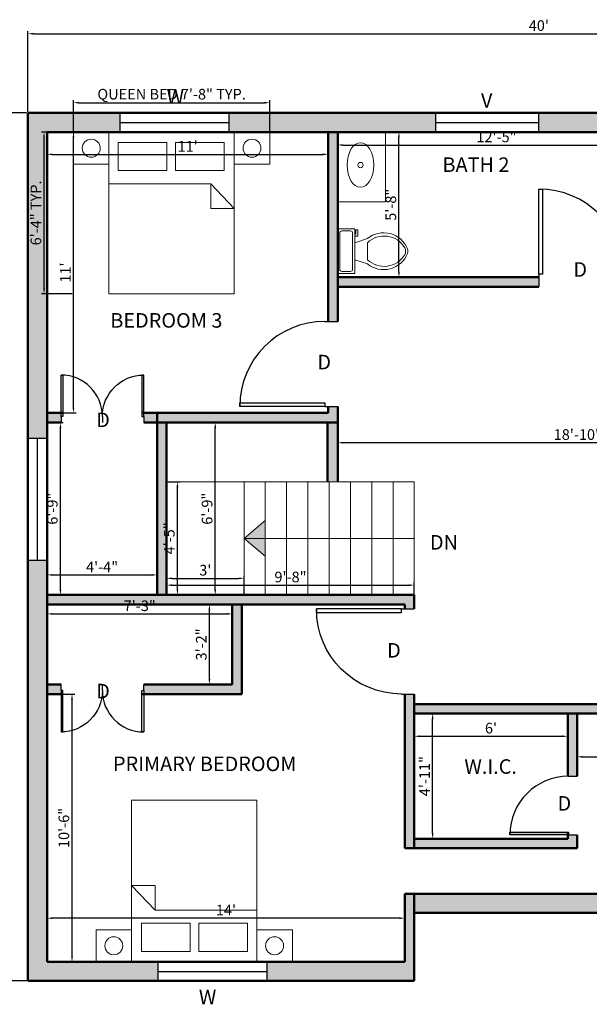
# Model space of a CAD drawing. Units: inches. Extents: x 1838 to 3464, y 573 to 2547.
# Tile 4 of 6: x 2788 to 3055, y 1325 to 1788. Entities that reach past the tile are written whole.
import ezdxf

# ---------------------------------------------------------------- set-up
doc = ezdxf.new("R2010")
doc.units = ezdxf.units.IN
for name, color, linetype, lineweight in [('A-ANNO-DIMS', 2, 'Continuous', 18), ('A-ANNO-TEXT', 7, 'Continuous', 18), ('A-AREA-IDEN', 3, 'Continuous', 18), ('A-DOOR', 4, 'Continuous', 25), ('A-FLOR-FIXT', 9, 'Continuous', 18), ('A-FLOR-STRS', 2, 'Continuous', 18), ('A-FURN', 8, 'Continuous', 18), ('A-GLAZ', 3, 'Continuous', 25), ('A-WALL', 1, 'Continuous', 50), ('A-WALL-PATT', 8, 'Continuous', 13)]:
    doc.layers.add(name, color=color, linetype=linetype, lineweight=lineweight)
doc.styles.get("Standard").update_dxf_attribs({"font": 'arial.ttf'})
doc.dimstyles.new('ISO-25', dxfattribs={"dimtxt": 5, "dimasz": 2.5, "dimexe": 1.25, "dimexo": 0.625, "dimtad": 1, "dimdec": 0, "dimlunit": 4, "dimtxsty": 'Standard', "dimcen": 2.5, "dimadec": 0, "dimazin": 0, "dimtfac": 1, "dimtdec": 0, "dimtmove": 0, "dimatfit": 3, "dimfxl": 1, "dimarcsym": 0})

# ---------------------------------------------------------------- blocks, each defined once
blk = doc.blocks.new('*U2')
for p, q in [((0, 0), (0, -6)), ((40, 0), (40, -6))]:
    blk.add_line(p, q)
blk.add_lwpolyline([(0, 0), (0, 40), (1.75, 40), (1.75, 0)], close=True)
blk.add_arc((0, 0), 40, 0, 90)
blk = doc.blocks.new('*U4')
for p, q in [((9.5, -6), (9.5, -2)), ((-10, -8.5), (-8, -8.5)), ((-10, -9.5), (-10, -8.5)), ((-8, -8.5), (-8, -8)), ((-7, -8), (-7, -9.5)), ((-4, -8), (-6, -14)), ((4, -8), (6, -14)), ((-7, -9.5), (-10, -9.5)), ((4, -14), (-4, -14))]:
    blk.add_line(p, q)
blk.add_lwpolyline([(10.5, -8), (10.5, 0), (-10.5, 0), (-10.5, -8)], close=True)
for points in [[(-9.5, -2), (-9.5, -6)], [(8.5, -1), (-8.5, -1)], [(-8.5, -7), (8.5, -7)]]:
    blk.add_lwpolyline(points)
for centre, radius, start, end in [((-8.62, -1.88), 0.884, 81.8699, 188.1301), ((8.62, -1.88), 0.884, 351.8699, 98.1301), ((-8.62, -6.12), 0.884, 171.8699, 278.1301), ((8.62, -6.12), 0.884, 261.8699, 8.1301), ((3.52, -21.58), 12.17, 141.4691, 247.9714), ((4.2, -21.82), 11.33, 136.3677, 238.9468), ((-3.52, -21.58), 12.17, 292.0284, 38.5307), ((-4.2, -21.82), 11.33, 301.053, 43.6321), ((0, -27.88), 4, 245.7318, 294.2682), ((0, -29), 4, 254.8605, 285.1395)]:
    blk.add_arc(centre, radius, start, end)
blk = doc.blocks.new('*D22')
at = {"layer": 'A-ANNO-DIMS', "color": 0, "lineweight": -2, "transparency": 16777216}
for p, q in [((2800.52, 1734.46), (2800.52, 1723.39)), ((2932.52, 1734.46), (2932.52, 1723.39)), ((2803.02, 1724.64), (2930.02, 1724.64))]:
    blk.add_line(p, q, dxfattribs=at)
at = {"layer": 'A-ANNO-DIMS', "color": 0, "lineweight": 100, "transparency": 16777216}
for points in [[(2803.02, 1725.06), (2803.02, 1724.23), (2800.52, 1724.64)], [(2930.02, 1725.06), (2930.02, 1724.23), (2932.52, 1724.64)]]:
    blk.add_solid(points, dxfattribs=at)
at = {"layer": 'Defpoints', "color": 0, "lineweight": 100, "transparency": 16777216}
for p in [(2800.52, 1735.09), (2932.52, 1735.09), (2932.52, 1724.64)]:
    blk.add_point(p, dxfattribs=at)
at = {"layer": 'A-ANNO-DIMS', "color": 0, "transparency": 16777216, "insert": (2866.52, 1727.78), "char_height": 5, "attachment_point": 5}
blk.add_mtext("11'", dxfattribs=at)
blk = doc.blocks.new('*D23')
at = {"layer": 'A-ANNO-DIMS', "color": 0, "lineweight": -2, "transparency": 16777216}
for p, q in [((2801.15, 1735.09), (2814.15, 1735.09)), ((2812.9, 1605.59), (2812.9, 1732.59)), ((2801.15, 1603.09), (2814.15, 1603.09))]:
    blk.add_line(p, q, dxfattribs=at)
at = {"layer": 'A-ANNO-DIMS', "color": 0, "lineweight": 100, "transparency": 16777216}
for points in [[(2812.48, 1732.59), (2813.32, 1732.59), (2812.9, 1735.09)], [(2812.48, 1605.59), (2813.32, 1605.59), (2812.9, 1603.09)]]:
    blk.add_solid(points, dxfattribs=at)
at = {"layer": 'Defpoints', "color": 0, "lineweight": 100, "transparency": 16777216}
for p in [(2800.52, 1735.09), (2812.9, 1735.09), (2800.52, 1603.09)]:
    blk.add_point(p, dxfattribs=at)
at = {"layer": 'A-ANNO-DIMS', "color": 0, "transparency": 16777216, "insert": (2809.77, 1669.09), "char_height": 5, "attachment_point": 5, "rotation": 90}
blk.add_mtext("11'", dxfattribs=at)
blk = doc.blocks.new('*D24')
at = {"layer": 'A-ANNO-DIMS', "color": 0, "lineweight": -2, "transparency": 16777216}
for p, q in [((2937.02, 1734.46), (2937.02, 1727.78)), ((3086.23, 1734.46), (3086.23, 1727.78)), ((2939.52, 1729.03), (3083.73, 1729.03))]:
    blk.add_line(p, q, dxfattribs=at)
at = {"layer": 'A-ANNO-DIMS', "color": 0, "lineweight": 100, "transparency": 16777216}
for points in [[(2939.52, 1729.44), (2939.52, 1728.61), (2937.02, 1729.03)], [(3083.73, 1729.44), (3083.73, 1728.61), (3086.23, 1729.03)]]:
    blk.add_solid(points, dxfattribs=at)
at = {"layer": 'Defpoints', "color": 0, "lineweight": 100, "transparency": 16777216}
for p in [(2937.02, 1735.09), (3086.23, 1735.09), (3086.23, 1729.03)]:
    blk.add_point(p, dxfattribs=at)
at = {"layer": 'A-ANNO-DIMS', "color": 0, "transparency": 16777216, "insert": (3011.63, 1732.2), "char_height": 5, "attachment_point": 5}
blk.add_mtext('12\'-5"', dxfattribs=at)
blk = doc.blocks.new('*D25')
at = {"layer": 'A-ANNO-DIMS', "color": 0, "lineweight": -2, "transparency": 16777216}
for p, q in [((2937.65, 1735.09), (2967.05, 1735.09)), ((2965.8, 1669.34), (2965.8, 1732.59)), ((2937.65, 1666.84), (2967.05, 1666.84))]:
    blk.add_line(p, q, dxfattribs=at)
at = {"layer": 'A-ANNO-DIMS', "color": 0, "lineweight": 100, "transparency": 16777216}
for points in [[(2965.39, 1732.59), (2966.22, 1732.59), (2965.8, 1735.09)], [(2965.39, 1669.34), (2966.22, 1669.34), (2965.8, 1666.84)]]:
    blk.add_solid(points, dxfattribs=at)
at = {"layer": 'Defpoints', "color": 0, "lineweight": 100, "transparency": 16777216}
for p in [(2937.02, 1735.09), (2965.8, 1735.09), (2937.02, 1666.84)]:
    blk.add_point(p, dxfattribs=at)
at = {"layer": 'A-ANNO-DIMS', "color": 0, "transparency": 16777216, "insert": (2962.63, 1700.96), "char_height": 5, "attachment_point": 5, "rotation": 90}
blk.add_mtext('5\'-8"', dxfattribs=at)
blk = doc.blocks.new('*D36')
at = {"layer": 'A-ANNO-DIMS', "color": 0, "lineweight": -2, "transparency": 16777216}
for p, q in [((3049.57, 1461.14), (3049.57, 1440.21)), ((3192.62, 1461.14), (3192.62, 1440.21)), ((3052.07, 1441.46), (3190.12, 1441.46))]:
    blk.add_line(p, q, dxfattribs=at)
at = {"layer": 'A-ANNO-DIMS', "color": 0, "lineweight": 100, "transparency": 16777216}
for points in [[(3052.07, 1441.87), (3052.07, 1441.04), (3049.57, 1441.46)], [(3190.12, 1441.87), (3190.12, 1441.04), (3192.62, 1441.46)]]:
    blk.add_solid(points, dxfattribs=at)
at = {"layer": 'Defpoints', "color": 0, "lineweight": 100, "transparency": 16777216}
for p in [(3049.57, 1461.77), (3192.62, 1461.77), (3192.62, 1441.46)]:
    blk.add_point(p, dxfattribs=at)
at = {"layer": 'A-ANNO-DIMS', "color": 0, "transparency": 16777216, "insert": (3121.09, 1444.59), "char_height": 5, "attachment_point": 5}
blk.add_mtext('11\'-11"', dxfattribs=at)
blk = doc.blocks.new('*D38')
at = {"layer": 'A-ANNO-DIMS', "color": 0, "lineweight": -2, "transparency": 16777216}
for p, q in [((2973.02, 1461.14), (2973.02, 1449.87)), ((3045.07, 1461.14), (3045.07, 1449.87)), ((2975.52, 1451.12), (3042.57, 1451.12))]:
    blk.add_line(p, q, dxfattribs=at)
at = {"layer": 'A-ANNO-DIMS', "color": 0, "lineweight": 100, "transparency": 16777216}
for points in [[(2975.52, 1451.53), (2975.52, 1450.7), (2973.02, 1451.12)], [(3042.57, 1451.53), (3042.57, 1450.7), (3045.07, 1451.12)]]:
    blk.add_solid(points, dxfattribs=at)
at = {"layer": 'Defpoints', "color": 0, "lineweight": 100, "transparency": 16777216}
for p in [(2973.02, 1461.77), (3045.07, 1461.77), (3045.07, 1451.12)]:
    blk.add_point(p, dxfattribs=at)
at = {"layer": 'A-ANNO-DIMS', "color": 0, "transparency": 16777216, "insert": (3009.05, 1454.3), "char_height": 5, "attachment_point": 5}
blk.add_mtext("6'", dxfattribs=at)
blk = doc.blocks.new('*D39')
at = {"layer": 'A-ANNO-DIMS', "color": 0, "lineweight": -2, "transparency": 16777216}
for p, q in [((2973.65, 1461.77), (2982.89, 1461.77)), ((2981.64, 1405.48), (2981.64, 1459.27)), ((2973.65, 1402.98), (2982.89, 1402.98))]:
    blk.add_line(p, q, dxfattribs=at)
at = {"layer": 'A-ANNO-DIMS', "color": 0, "lineweight": 100, "transparency": 16777216}
for points in [[(2981.22, 1459.27), (2982.05, 1459.27), (2981.64, 1461.77)], [(2981.22, 1405.48), (2982.05, 1405.48), (2981.64, 1402.98)]]:
    blk.add_solid(points, dxfattribs=at)
at = {"layer": 'Defpoints', "color": 0, "lineweight": 100, "transparency": 16777216}
for p in [(2973.02, 1461.77), (2981.64, 1461.77), (2973.02, 1402.98)]:
    blk.add_point(p, dxfattribs=at)
at = {"layer": 'A-ANNO-DIMS', "color": 0, "transparency": 16777216, "insert": (2978.5, 1432.37), "char_height": 5, "attachment_point": 5, "rotation": 90}
blk.add_mtext('4\'-11"', dxfattribs=at)
blk = doc.blocks.new('*D40')
at = {"layer": 'A-ANNO-DIMS', "color": 0, "lineweight": -2, "transparency": 16777216}
for p, q in [((2800.52, 1345.71), (2800.52, 1366.86)), ((2966.02, 1365.61), (2803.02, 1365.61)), ((2968.52, 1345.71), (2968.52, 1366.86))]:
    blk.add_line(p, q, dxfattribs=at)
at = {"layer": 'A-ANNO-DIMS', "color": 0, "lineweight": 100, "transparency": 16777216}
for points in [[(2803.02, 1366.03), (2803.02, 1365.2), (2800.52, 1365.61)], [(2966.02, 1366.03), (2966.02, 1365.2), (2968.52, 1365.61)]]:
    blk.add_solid(points, dxfattribs=at)
at = {"layer": 'Defpoints', "color": 0, "lineweight": 100, "transparency": 16777216}
for p in [(2800.52, 1365.61), (2800.52, 1345.09), (2968.52, 1345.09)]:
    blk.add_point(p, dxfattribs=at)
at = {"layer": 'A-ANNO-DIMS', "color": 0, "transparency": 16777216, "insert": (2884.52, 1368.75), "char_height": 5, "attachment_point": 5}
blk.add_mtext("14'", dxfattribs=at)
blk = doc.blocks.new('*D41')
at = {"layer": 'A-ANNO-DIMS', "color": 0, "lineweight": -2, "transparency": 16777216}
for p, q in [((2801.15, 1470.97), (2813.47, 1470.97)), ((2812.22, 1347.59), (2812.22, 1468.47)), ((2801.15, 1345.09), (2813.47, 1345.09))]:
    blk.add_line(p, q, dxfattribs=at)
at = {"layer": 'A-ANNO-DIMS', "color": 0, "lineweight": 100, "transparency": 16777216}
for points in [[(2811.8, 1468.47), (2812.64, 1468.47), (2812.22, 1470.97)], [(2811.8, 1347.59), (2812.64, 1347.59), (2812.22, 1345.09)]]:
    blk.add_solid(points, dxfattribs=at)
at = {"layer": 'Defpoints', "color": 0, "lineweight": 100, "transparency": 16777216}
for p in [(2800.52, 1470.97), (2812.22, 1470.97), (2800.52, 1345.09)]:
    blk.add_point(p, dxfattribs=at)
at = {"layer": 'A-ANNO-DIMS', "color": 0, "transparency": 16777216, "insert": (2809.04, 1408.03), "char_height": 5, "attachment_point": 5, "rotation": 90}
blk.add_mtext('10\'-6"', dxfattribs=at)
blk = doc.blocks.new('*D42')
at = {"layer": 'A-ANNO-DIMS', "color": 0, "lineweight": -2, "transparency": 16777216}
for p, q in [((2800.52, 1512.46), (2800.52, 1507.38)), ((2887.51, 1512.46), (2887.51, 1507.38)), ((2803.02, 1508.63), (2885.01, 1508.63))]:
    blk.add_line(p, q, dxfattribs=at)
at = {"layer": 'A-ANNO-DIMS', "color": 0, "lineweight": 100, "transparency": 16777216}
for points in [[(2803.02, 1509.05), (2803.02, 1508.22), (2800.52, 1508.63)], [(2885.01, 1509.05), (2885.01, 1508.22), (2887.51, 1508.63)]]:
    blk.add_solid(points, dxfattribs=at)
at = {"layer": 'Defpoints', "color": 0, "lineweight": 100, "transparency": 16777216}
for p in [(2800.52, 1513.09), (2887.51, 1513.09), (2887.51, 1508.63)]:
    blk.add_point(p, dxfattribs=at)
at = {"layer": 'A-ANNO-DIMS', "color": 0, "transparency": 16777216, "insert": (2844.02, 1511.81), "char_height": 5, "attachment_point": 5}
blk.add_mtext('7\'-3"', dxfattribs=at)
blk = doc.blocks.new('*D43')
at = {"layer": 'A-ANNO-DIMS', "color": 0, "lineweight": -2, "transparency": 16777216}
for p, q in [((2886.88, 1513.09), (2875.52, 1513.09)), ((2876.77, 1477.97), (2876.77, 1510.59)), ((2886.88, 1475.47), (2875.52, 1475.47))]:
    blk.add_line(p, q, dxfattribs=at)
at = {"layer": 'A-ANNO-DIMS', "color": 0, "lineweight": 100, "transparency": 16777216}
for points in [[(2876.36, 1510.59), (2877.19, 1510.59), (2876.77, 1513.09)], [(2876.36, 1477.97), (2877.19, 1477.97), (2876.77, 1475.47)]]:
    blk.add_solid(points, dxfattribs=at)
at = {"layer": 'Defpoints', "color": 0, "lineweight": 100, "transparency": 16777216}
for p in [(2876.77, 1513.09), (2887.51, 1513.09), (2887.51, 1475.47)]:
    blk.add_point(p, dxfattribs=at)
at = {"layer": 'A-ANNO-DIMS', "color": 0, "transparency": 16777216, "insert": (2873.59, 1494.28), "char_height": 5, "attachment_point": 5, "rotation": 90}
blk.add_mtext('3\'-2"', dxfattribs=at)
blk = doc.blocks.new('*D44')
at = {"layer": 'A-ANNO-DIMS', "color": 0, "lineweight": -2, "transparency": 16777216}
for p, q in [((2800.52, 1518.21), (2800.52, 1528.2)), ((2852.18, 1518.21), (2852.18, 1528.2)), ((2803.02, 1526.95), (2849.68, 1526.95))]:
    blk.add_line(p, q, dxfattribs=at)
at = {"layer": 'A-ANNO-DIMS', "color": 0, "lineweight": 100, "transparency": 16777216}
for points in [[(2803.02, 1527.37), (2803.02, 1526.54), (2800.52, 1526.95)], [(2849.68, 1527.37), (2849.68, 1526.54), (2852.18, 1526.95)]]:
    blk.add_solid(points, dxfattribs=at)
at = {"layer": 'Defpoints', "color": 0, "lineweight": 100, "transparency": 16777216}
for p in [(2852.18, 1526.95), (2800.52, 1517.59), (2852.18, 1517.59)]:
    blk.add_point(p, dxfattribs=at)
at = {"layer": 'A-ANNO-DIMS', "color": 0, "transparency": 16777216, "insert": (2826.35, 1530.08), "char_height": 5, "attachment_point": 5}
blk.add_mtext('4\'-4"', dxfattribs=at)
blk = doc.blocks.new('*D45')
at = {"layer": 'A-ANNO-DIMS', "color": 0, "lineweight": -2, "transparency": 16777216}
for p, q in [((2801.15, 1598.59), (2808.03, 1598.59)), ((2806.78, 1520.09), (2806.78, 1596.09)), ((2801.15, 1517.59), (2808.03, 1517.59))]:
    blk.add_line(p, q, dxfattribs=at)
at = {"layer": 'A-ANNO-DIMS', "color": 0, "lineweight": 100, "transparency": 16777216}
for points in [[(2806.37, 1596.09), (2807.2, 1596.09), (2806.78, 1598.59)], [(2806.37, 1520.09), (2807.2, 1520.09), (2806.78, 1517.59)]]:
    blk.add_solid(points, dxfattribs=at)
at = {"layer": 'Defpoints', "color": 0, "lineweight": 100, "transparency": 16777216}
for p in [(2800.52, 1598.59), (2806.78, 1598.59), (2800.52, 1517.59)]:
    blk.add_point(p, dxfattribs=at)
at = {"layer": 'A-ANNO-DIMS', "color": 0, "transparency": 16777216, "insert": (2803.6, 1558.09), "char_height": 5, "attachment_point": 5, "rotation": 90}
blk.add_mtext('6\'-9"', dxfattribs=at)
blk = doc.blocks.new('*D46')
at = {"layer": 'A-ANNO-DIMS', "color": 0, "lineweight": -2, "transparency": 16777216}
for p, q in [((2856.68, 1518.21), (2856.68, 1523.4)), ((2973.02, 1518.21), (2973.02, 1523.4)), ((2859.18, 1522.15), (2970.52, 1522.15))]:
    blk.add_line(p, q, dxfattribs=at)
at = {"layer": 'A-ANNO-DIMS', "color": 0, "lineweight": 100, "transparency": 16777216}
for points in [[(2859.18, 1522.57), (2859.18, 1521.74), (2856.68, 1522.15)], [(2970.52, 1522.57), (2970.52, 1521.74), (2973.02, 1522.15)]]:
    blk.add_solid(points, dxfattribs=at)
at = {"layer": 'Defpoints', "color": 0, "lineweight": 100, "transparency": 16777216}
for p in [(2973.02, 1522.15), (2856.68, 1517.59), (2973.02, 1517.59)]:
    blk.add_point(p, dxfattribs=at)
at = {"layer": 'A-ANNO-DIMS', "color": 0, "transparency": 16777216, "insert": (2914.85, 1525.33), "char_height": 5, "attachment_point": 5}
blk.add_mtext('9\'-8"', dxfattribs=at)
blk = doc.blocks.new('*D47')
at = {"layer": 'A-ANNO-DIMS', "color": 0, "lineweight": -2, "transparency": 16777216}
for p, q in [((2857.31, 1598.59), (2880.75, 1598.59)), ((2879.5, 1520.09), (2879.5, 1596.09)), ((2857.31, 1517.59), (2880.75, 1517.59))]:
    blk.add_line(p, q, dxfattribs=at)
at = {"layer": 'A-ANNO-DIMS', "color": 0, "lineweight": 100, "transparency": 16777216}
for points in [[(2879.08, 1596.09), (2879.92, 1596.09), (2879.5, 1598.59)], [(2879.08, 1520.09), (2879.92, 1520.09), (2879.5, 1517.59)]]:
    blk.add_solid(points, dxfattribs=at)
at = {"layer": 'Defpoints', "color": 0, "lineweight": 100, "transparency": 16777216}
for p in [(2856.68, 1598.59), (2879.5, 1598.59), (2856.68, 1517.59)]:
    blk.add_point(p, dxfattribs=at)
at = {"layer": 'A-ANNO-DIMS', "color": 0, "transparency": 16777216, "insert": (2876.32, 1558.09), "char_height": 5, "attachment_point": 5, "rotation": 90}
blk.add_mtext('6\'-9"', dxfattribs=at)
blk = doc.blocks.new('*D48')
at = {"layer": 'A-ANNO-DIMS', "color": 0, "lineweight": -2, "transparency": 16777216}
for p, q in [((2857.31, 1570.68), (2862.98, 1570.68)), ((2861.73, 1520.09), (2861.73, 1568.18)), ((2857.31, 1517.59), (2862.98, 1517.59))]:
    blk.add_line(p, q, dxfattribs=at)
at = {"layer": 'A-ANNO-DIMS', "color": 0, "lineweight": 100, "transparency": 16777216}
for points in [[(2861.32, 1568.18), (2862.15, 1568.18), (2861.73, 1570.68)], [(2861.32, 1520.09), (2862.15, 1520.09), (2861.73, 1517.59)]]:
    blk.add_solid(points, dxfattribs=at)
at = {"layer": 'Defpoints', "color": 0, "lineweight": 100, "transparency": 16777216}
for p in [(2856.68, 1570.68), (2861.73, 1570.68), (2856.68, 1517.59)]:
    blk.add_point(p, dxfattribs=at)
at = {"layer": 'A-ANNO-DIMS', "color": 0, "transparency": 16777216, "insert": (2858.57, 1544.13), "char_height": 5, "attachment_point": 5, "rotation": 90}
blk.add_mtext('4\'-5"', dxfattribs=at)
blk = doc.blocks.new('*D49')
at = {"layer": 'A-ANNO-DIMS', "color": 0, "lineweight": -2, "transparency": 16777216}
for p, q in [((2856.68, 1518.21), (2856.68, 1526.59)), ((2859.18, 1525.34), (2890.52, 1525.34)), ((2893.02, 1518.21), (2893.02, 1526.59))]:
    blk.add_line(p, q, dxfattribs=at)
at = {"layer": 'A-ANNO-DIMS', "color": 0, "lineweight": 100, "transparency": 16777216}
for points in [[(2859.18, 1525.76), (2859.18, 1524.93), (2856.68, 1525.34)], [(2890.52, 1525.76), (2890.52, 1524.93), (2893.02, 1525.34)]]:
    blk.add_solid(points, dxfattribs=at)
at = {"layer": 'Defpoints', "color": 0, "lineweight": 100, "transparency": 16777216}
for p in [(2893.02, 1525.34), (2856.68, 1517.59), (2893.02, 1517.59)]:
    blk.add_point(p, dxfattribs=at)
at = {"layer": 'A-ANNO-DIMS', "color": 0, "transparency": 16777216, "insert": (2874.85, 1528.52), "char_height": 5, "attachment_point": 5}
blk.add_mtext("3'", dxfattribs=at)
blk = doc.blocks.new('*D50')
at = {"layer": 'A-ANNO-DIMS', "color": 0, "lineweight": -2, "transparency": 16777216}
for p, q in [((2937.02, 1597.96), (2937.02, 1587.86)), ((3162.64, 1597.96), (3162.64, 1587.86)), ((3160.14, 1589.11), (2939.52, 1589.11))]:
    blk.add_line(p, q, dxfattribs=at)
at = {"layer": 'A-ANNO-DIMS', "color": 0, "lineweight": 100, "transparency": 16777216}
for points in [[(2939.52, 1589.52), (2939.52, 1588.69), (2937.02, 1589.11)], [(3160.14, 1589.52), (3160.14, 1588.69), (3162.64, 1589.11)]]:
    blk.add_solid(points, dxfattribs=at)
at = {"layer": 'Defpoints', "color": 0, "lineweight": 100, "transparency": 16777216}
for p in [(2937.02, 1598.59), (3162.64, 1598.59), (2937.02, 1589.11)]:
    blk.add_point(p, dxfattribs=at)
at = {"layer": 'A-ANNO-DIMS', "color": 0, "transparency": 16777216, "insert": (3049.83, 1592.29), "char_height": 5, "attachment_point": 5}
blk.add_mtext('18\'-10"', dxfattribs=at)
blk = doc.blocks.new('*D65')
at = {"layer": 'A-ANNO-DIMS', "color": 0, "lineweight": -2, "transparency": 16777216}
for p, q in [((2791.52, 1744.71), (2791.52, 1782.6)), ((3271.52, 1744.71), (3271.52, 1782.6)), ((2794.02, 1781.35), (3269.02, 1781.35))]:
    blk.add_line(p, q, dxfattribs=at)
at = {"layer": 'A-ANNO-DIMS', "color": 0, "lineweight": 100, "transparency": 16777216}
for points in [[(2794.02, 1781.77), (2794.02, 1780.94), (2791.52, 1781.35)], [(3269.02, 1781.77), (3269.02, 1780.94), (3271.52, 1781.35)]]:
    blk.add_solid(points, dxfattribs=at)
at = {"layer": 'Defpoints', "color": 0, "lineweight": 100, "transparency": 16777216}
for p in [(3271.52, 1781.35), (2791.52, 1744.09), (3271.52, 1744.09)]:
    blk.add_point(p, dxfattribs=at)
at = {"layer": 'A-ANNO-DIMS', "color": 0, "transparency": 16777216, "insert": (3031.52, 1784.53), "char_height": 5, "attachment_point": 5}
blk.add_mtext("40'", dxfattribs=at)
blk = doc.blocks.new('*D66')
at = {"layer": 'A-ANNO-DIMS', "color": 0, "lineweight": -2, "transparency": 16777216}
for p, q in [((2790.9, 1744.09), (2755.73, 1744.09)), ((2756.98, 1338.59), (2756.98, 1741.59)), ((2790.9, 1336.09), (2755.73, 1336.09))]:
    blk.add_line(p, q, dxfattribs=at)
at = {"layer": 'A-ANNO-DIMS', "color": 0, "lineweight": 100, "transparency": 16777216}
for points in [[(2756.56, 1741.59), (2757.39, 1741.59), (2756.98, 1744.09)], [(2756.56, 1338.59), (2757.39, 1338.59), (2756.98, 1336.09)]]:
    blk.add_solid(points, dxfattribs=at)
at = {"layer": 'Defpoints', "color": 0, "lineweight": 100, "transparency": 16777216}
for p in [(2756.98, 1744.09), (2791.52, 1744.09), (2791.52, 1336.09)]:
    blk.add_point(p, dxfattribs=at)
at = {"layer": 'A-ANNO-DIMS', "color": 0, "transparency": 16777216, "insert": (2753.8, 1540.09), "char_height": 5, "attachment_point": 5, "rotation": 90}
blk.add_mtext("34'", dxfattribs=at)
blk = doc.blocks.new('BED-QUEEN')
for p, q in [((2829.57, 1710.8), (2877.39, 1710.8)), ((2877.39, 1710.8), (2877.39, 1699.19)), ((2888.43, 1699.19), (2877.39, 1710.8)), ((2877.39, 1699.19), (2888.43, 1699.19))]:
    blk.add_line(p, q)
for points in [[(2829.57, 1735.09), (2812.9, 1735.09), (2812.9, 1719.98), (2829.57, 1719.98)], [(2829.57, 1735.09), (2888.43, 1735.09), (2888.43, 1659.13), (2829.57, 1659.13)], [(2905.11, 1735.09), (2888.43, 1735.09), (2888.43, 1719.98), (2905.11, 1719.98)]]:
    blk.add_lwpolyline(points, close=True)
for centre in [(2821.24, 1727.53), (2896.77, 1727.53)]:
    blk.add_circle(centre, 4.22)
blk = doc.blocks.new('*D68')
at = {"layer": 'A-ANNO-DIMS', "color": 0, "lineweight": -2, "transparency": 16777216}
for p, q in [((2812.9, 1735.71), (2812.9, 1750.17)), ((2905.11, 1735.71), (2905.11, 1750.17)), ((2815.4, 1748.92), (2902.61, 1748.92))]:
    blk.add_line(p, q, dxfattribs=at)
at = {"layer": 'A-ANNO-DIMS', "color": 0, "lineweight": 100, "transparency": 16777216}
for points in [[(2815.4, 1749.33), (2815.4, 1748.5), (2812.9, 1748.92)], [(2902.61, 1749.33), (2902.61, 1748.5), (2905.11, 1748.92)]]:
    blk.add_solid(points, dxfattribs=at)
at = {"layer": 'Defpoints', "color": 0, "lineweight": 100, "transparency": 16777216}
for p in [(2905.11, 1748.92), (2812.9, 1735.09), (2905.11, 1735.09)]:
    blk.add_point(p, dxfattribs=at)
at = {"layer": 'A-ANNO-DIMS', "color": 0, "transparency": 16777216, "insert": (2859, 1752.28), "char_height": 5, "attachment_point": 5}
blk.add_mtext('QUEEN BED 7\'-8" TYP.', dxfattribs=at)
blk = doc.blocks.new('*D69')
at = {"layer": 'A-ANNO-DIMS', "color": 0, "lineweight": -2, "transparency": 16777216}
for p, q in [((2812.28, 1735.09), (2797.82, 1735.09)), ((2799.07, 1661.63), (2799.07, 1732.59)), ((2812.28, 1659.13), (2797.82, 1659.13))]:
    blk.add_line(p, q, dxfattribs=at)
at = {"layer": 'A-ANNO-DIMS', "color": 0, "lineweight": 100, "transparency": 16777216}
for points in [[(2798.65, 1732.59), (2799.49, 1732.59), (2799.07, 1735.09)], [(2798.65, 1661.63), (2799.49, 1661.63), (2799.07, 1659.13)]]:
    blk.add_solid(points, dxfattribs=at)
at = {"layer": 'Defpoints', "color": 0, "lineweight": 100, "transparency": 16777216}
for p in [(2799.07, 1735.09), (2812.9, 1735.09), (2812.9, 1659.13)]:
    blk.add_point(p, dxfattribs=at)
at = {"layer": 'A-ANNO-DIMS', "color": 0, "transparency": 16777216, "insert": (2795.89, 1697.11), "char_height": 5, "attachment_point": 5, "rotation": 90}
blk.add_mtext('6\'-4" TYP.', dxfattribs=at)

msp = doc.modelspace()

# ---------------------------------------------------------------- hatches: boundary and pattern name
at = {"layer": 'A-FLOR-STRS'}
h = msp.add_hatch(color=256, dxfattribs=at)
h.dxf.hatch_style = 1
h.paths.add_polyline_path([(2903.02, 1552.5), (2893.02, 1544.13), (2903.02, 1544.13)])
h.paths.add_polyline_path([(2903.02, 1544.13), (2893.02, 1544.13), (2903.02, 1535.77)])
at = {"layer": 'A-WALL-PATT'}
h = msp.add_hatch(color=256, dxfattribs=at)
h.dxf.hatch_style = 1
h.paths.add_polyline_path([(2800.52, 1735.09), (2834.76, 1735.09), (2834.76, 1744.09), (2791.52, 1744.09), (2791.52, 1591.27), (2800.52, 1591.27)])
h.paths.add_polyline_path([(2982.96, 1744.09), (2885.93, 1744.09), (2885.93, 1735.09), (2888.43, 1735.09), (2932.52, 1735.09), (2982.96, 1735.09)])
h.paths.add_polyline_path([(3199.72, 1744.09), (3031.52, 1744.09), (3031.52, 1735.09), (3199.72, 1735.09)])
h.paths.add_polyline_path([(3271.52, 1744.09), (3250.89, 1744.09), (3250.89, 1735.09), (3262.52, 1735.09), (3262.52, 1573.47), (3271.52, 1573.47)])
h.paths.add_polyline_path([(3262.52, 1603.09), (3130.52, 1603.09), (3130.52, 1607.14), (3126.02, 1607.14), (3126.02, 1598.59), (3262.52, 1598.59)])
h.paths.add_polyline_path([(3130.52, 1666.84), (3122.07, 1666.84), (3122.07, 1679.27), (3120.48, 1679.27), (3117.57, 1679.27), (3117.57, 1666.84), (3071.52, 1666.84), (3071.52, 1662.34), (3126.02, 1662.34), (3126.02, 1647.14), (3130.52, 1647.14)])
h.paths.add_polyline_path([(3122.07, 1735.09), (3117.57, 1735.09), (3117.57, 1718.07), (3120.48, 1718.07), (3122.07, 1718.07)])
h.paths.add_polyline_path([(3090.73, 1735.09), (3086.23, 1735.09), (3086.23, 1666.84), (3090.73, 1666.84)])
h.paths.add_polyline_path([(3031.52, 1666.84), (2937.02, 1666.84), (2937.02, 1662.34), (3031.52, 1662.34)])
h.paths.add_polyline_path([(2937.02, 1735.09), (2932.52, 1735.09), (2932.52, 1646.12), (2937.02, 1646.12)])
h.paths.add_polyline_path([(2937.02, 1606.12), (2932.52, 1606.12), (2932.52, 1603.09), (2852.18, 1603.09), (2852.18, 1598.59), (2937.02, 1598.59)])
h.paths.add_polyline_path([(2852.18, 1603.09), (2845.88, 1603.09), (2845.88, 1601.49), (2845.88, 1598.59), (2852.18, 1598.59)])
h.paths.add_polyline_path([(2807.08, 1601.49), (2807.08, 1603.09), (2800.52, 1603.09), (2800.52, 1598.59), (2807.08, 1598.59)], flags=17)
h.paths.add_polyline_path([(2937.02, 1598.59), (2932.24, 1598.59), (2932.24, 1570.68), (2937.02, 1570.68)])
h.paths.add_polyline_path([(2800.52, 1513.09), (2800.52, 1533.8), (2791.52, 1533.8), (2791.52, 1336.09), (2852.63, 1336.09), (2852.63, 1345.09), (2840.19, 1345.09), (2823.52, 1345.09), (2800.52, 1345.09)])
h.paths.add_polyline_path([(2807.08, 1472.56), (2807.08, 1475.47), (2800.52, 1475.47), (2800.52, 1470.97), (2807.08, 1470.97)], flags=17)
h.paths.add_polyline_path([(2892.01, 1513.09), (2887.51, 1513.09), (2887.51, 1475.47), (2845.88, 1475.47), (2845.88, 1472.56), (2845.88, 1470.97), (2892.01, 1470.97)])
h.paths.add_polyline_path([(2973.02, 1517.59), (2800.52, 1517.59), (2800.52, 1513.09), (2968.52, 1513.09), (2968.52, 1510.98), (2973.02, 1510.98)])
h.paths.add_polyline_path([(2856.68, 1598.59), (2852.18, 1598.59), (2852.18, 1517.59), (2856.68, 1517.59)])
h.paths.add_polyline_path([(2973.02, 1376.09), (2973.02, 1377.09), (2968.52, 1377.09), (2968.52, 1345.09), (2903.8, 1345.09), (2903.8, 1336.09), (2973.02, 1336.09)])
h.paths.add_polyline_path([(3089.35, 1377.09), (2973.02, 1377.09), (2973.02, 1368.09), (3089.35, 1368.09)])
h.paths.add_polyline_path([(2973.02, 1470.98), (2968.52, 1470.98), (2968.52, 1398.48), (2973.02, 1398.48)])
h.paths.add_polyline_path([(3262.52, 1466.27), (2973.02, 1466.27), (2973.02, 1461.77), (3262.52, 1461.77)])
h.paths.add_polyline_path([(3017.96, 1406), (3045.44, 1406), (3045.44, 1404.8), (3017.93, 1404.8), (3017.93, 1406), (3017.96, 1406, -0.397522), (3045.07, 1432.31), (3045.07, 1461.77), (3049.57, 1461.77), (3049.57, 1432.31), (3045.44, 1432.31, 0.401453)])
h.paths.add_polyline_path([(3049.57, 1404.8), (3045.07, 1404.8), (3045.07, 1402.98), (2973.02, 1402.98), (2973.02, 1398.48), (3049.57, 1398.48)])
h.paths.add_polyline_path([(3271.52, 1422.39), (3262.52, 1422.39), (3262.52, 1377.09), (3143.98, 1377.09), (3143.98, 1368.09), (3271.52, 1368.09)])
h.paths.add_polyline_path([(3271.52, 1491.77), (3262.52, 1491.77), (3262.52, 1453.4), (3271.52, 1453.4)])
h.paths.add_polyline_path([(3167.14, 1542.08), (3162.64, 1542.08), (3162.64, 1466.27), (3167.14, 1466.27)])
h.paths.add_polyline_path([(3167.14, 1598.59), (3162.64, 1598.59), (3162.64, 1582.08), (3167.14, 1582.08)])

# ---------------------------------------------------------------- linework, layer by layer
at = {"layer": 'A-FLOR-FIXT'}
msp.add_lwpolyline([(2937.02, 1702.34), (2959.43, 1702.34), (2959.43, 1735.09), (2937.02, 1735.09)], close=True, dxfattribs=at)
msp.add_circle((2947.74, 1719.62), 1.25, dxfattribs=at)
msp.add_ellipse((2947.74, 1719.62), major_axis=(0, 10.44), ratio=0.604248, dxfattribs=at)
at = {"layer": 'A-FLOR-STRS'}
for p, q in [((2856.68, 1570.68), (2973.02, 1570.68)), ((2893.02, 1517.59), (2893.02, 1570.68)), ((2903.02, 1517.59), (2903.02, 1570.68)), ((2913.02, 1517.59), (2913.02, 1570.68)), ((2923.02, 1517.59), (2923.02, 1570.68)), ((2933.02, 1517.59), (2933.02, 1570.68)), ((2943.02, 1517.59), (2943.02, 1570.68)), ((2953.02, 1517.59), (2953.02, 1570.68)), ((2963.02, 1517.59), (2963.02, 1570.68)), ((2973.02, 1517.59), (2973.02, 1570.68)), ((2893.02, 1544.13), (2903.02, 1552.5)), ((2973.02, 1544.13), (2893.02, 1544.13)), ((2893.02, 1544.13), (2903.02, 1535.77))]:
    msp.add_line(p, q, dxfattribs=at)
at = {"layer": 'A-FURN'}
for points in [[(2833.9, 1730.28), (2856.77, 1730.28), (2856.77, 1716.98), (2833.9, 1716.98)], [(2860.89, 1730.28), (2883.76, 1730.28), (2883.76, 1716.98), (2860.89, 1716.98)], [(2867.73, 1349.89), (2844.86, 1349.89), (2844.86, 1363.19), (2867.73, 1363.19)], [(2894.72, 1349.89), (2871.85, 1349.89), (2871.85, 1363.19), (2894.72, 1363.19)]]:
    msp.add_lwpolyline(points, close=True, dxfattribs=at)
at = {"layer": 'A-GLAZ'}
for p, q in [((2834.76, 1739.59), (2885.93, 1739.59)), ((2982.96, 1739.59), (3031.52, 1739.59)), ((2796.02, 1533.8), (2796.02, 1591.27)), ((2852.63, 1340.59), (2903.8, 1340.59))]:
    msp.add_line(p, q, dxfattribs=at)
for points in [[(2834.76, 1744.09), (2885.93, 1744.09), (2885.93, 1735.09), (2834.76, 1735.09)], [(2982.96, 1735.09), (3031.52, 1735.09), (3031.52, 1744.09), (2982.96, 1744.09)], [(2800.52, 1533.8), (2791.52, 1533.8), (2791.52, 1591.27), (2800.52, 1591.27)], [(2852.63, 1345.09), (2903.8, 1345.09), (2903.8, 1336.09), (2852.63, 1336.09)]]:
    msp.add_lwpolyline(points, close=True, dxfattribs=at)
at = {"layer": 'A-WALL'}
for p, q in [((2791.52, 1744.09), (3271.52, 1744.09)), ((2791.52, 1336.09), (2791.52, 1744.09)), ((2800.52, 1735.09), (3262.52, 1735.09)), ((2800.52, 1345.09), (2800.52, 1735.09)), ((2800.52, 1735.09), (2932.52, 1735.09)), ((2932.52, 1735.09), (2932.52, 1646.12)), ((2937.02, 1735.09), (2937.02, 1646.12)), ((3031.52, 1666.84), (2937.02, 1666.84)), ((3031.52, 1662.34), (2937.02, 1662.34)), ((2932.52, 1606.12), (2932.52, 1603.09)), ((2937.02, 1606.12), (2937.02, 1598.59)), ((2807.93, 1603.09), (2800.52, 1603.09)), ((2826.55, 1603.09), (2826.41, 1603.09)), ((2932.52, 1603.09), (2845.03, 1603.09)), ((2852.18, 1598.59), (2852.18, 1603.09)), ((2807.08, 1598.59), (2800.52, 1598.59)), ((2937.02, 1598.59), (2845.88, 1598.59)), ((2852.18, 1517.59), (2852.18, 1598.59)), ((2856.68, 1517.59), (2856.68, 1598.59)), ((2932.24, 1598.59), (2932.24, 1570.68)), ((2937.02, 1598.59), (2937.02, 1570.68)), ((2856.68, 1570.68), (2856.68, 1570.68)), ((2800.52, 1517.59), (2973.02, 1517.59)), ((2973.02, 1517.59), (2973.02, 1510.98)), ((2800.52, 1345.09), (2800.52, 1513.09)), ((2800.52, 1513.09), (2968.52, 1513.09)), ((2887.51, 1513.09), (2887.51, 1475.47)), ((2892.01, 1513.09), (2892.01, 1470.97)), ((2968.52, 1513.09), (2968.52, 1510.98)), ((2807.08, 1475.47), (2800.52, 1475.47)), ((2887.51, 1475.47), (2845.88, 1475.47)), ((2807.93, 1470.97), (2800.52, 1470.97)), ((2826.55, 1470.97), (2826.41, 1470.97)), ((2892.01, 1470.97), (2845.03, 1470.97)), ((2968.52, 1470.98), (2968.52, 1398.48)), ((2973.02, 1470.98), (2973.02, 1398.48)), ((2973.02, 1466.27), (3262.52, 1466.27)), ((2973.02, 1461.77), (3262.52, 1461.77)), ((3045.07, 1461.77), (3045.07, 1432.31)), ((3049.57, 1461.77), (3049.57, 1432.31)), ((3045.07, 1402.98), (2973.02, 1402.98)), ((3045.07, 1406), (3045.07, 1402.98)), ((3049.57, 1404.8), (3049.57, 1398.48)), ((2973.02, 1398.48), (2968.52, 1398.48)), ((3049.57, 1398.48), (2973.02, 1398.48)), ((2973.02, 1377.09), (2968.52, 1377.09)), ((2968.52, 1377.09), (2968.52, 1345.09)), ((2973.02, 1345.09), (2973.02, 1377.09)), ((2973.02, 1377.09), (3262.52, 1377.09)), ((2973.02, 1377.09), (2973.02, 1345.09)), ((2973.02, 1336.09), (2973.02, 1376.09)), ((2973.02, 1368.09), (3271.52, 1368.09)), ((2968.52, 1345.09), (2800.52, 1345.09)), ((2973.02, 1336.09), (2791.52, 1336.09))]:
    msp.add_line(p, q, dxfattribs=at)

# ---------------------------------------------------------------- block references
at = {"layer": 'A-DOOR'}
msp.add_blockref('*U2', (3031.52, 1668.34), dxfattribs=at)
at = {"layer": 'A-DOOR', "rotation": 90}
msp.add_blockref('*U2', (2931.02, 1606.12), dxfattribs=at)
at = {"layer": 'A-DOOR', "yscale": 0.4849649576214688, "zscale": 0.4849649576214688}
for p, xscale in [((2807.08, 1601.49), 0.4849649576214688), ((2845.88, 1601.49), -0.4849649576214688)]:
    msp.add_blockref('*U2', p, dxfattribs=dict(at, xscale=xscale))
at = {"layer": 'A-DOOR', "xscale": -1, "rotation": 90}
msp.add_blockref('*U2', (2967.02, 1510.98), dxfattribs=at)
at = {"layer": 'A-DOOR'}
for p, xscale, yscale, zscale, rotation in [((2807.08, 1472.56), -0.4849649576214688, 0.4849649576214688, 0.4849649576214688, 180), ((2845.88, 1472.56), 0.4849649576214688, 0.4849649576214688, 0.4849649576214688, 180), ((3045.44, 1404.8), 0.6878342338658366, 0.6878342338658366, 0.6878342338658366, 90)]:
    msp.add_blockref('*U2', p, dxfattribs=dict(at, xscale=xscale, yscale=yscale, zscale=zscale, rotation=rotation))
at = {"layer": 'A-FLOR-FIXT', "xscale": -1, "rotation": 90}
msp.add_blockref('*U4', (2937.02, 1679.12), dxfattribs=at)
at = {"layer": 'A-FURN'}
msp.add_blockref('BED-QUEEN', (0, 0), dxfattribs=at)
at = {"layer": 'A-FURN', "rotation": 180}
msp.add_blockref('BED-QUEEN', (5728.62, 3080.17), dxfattribs=at)

# ---------------------------------------------------------------- texts
at = {"layer": 'A-ANNO-TEXT', "attachment_point": 1}
for s, insert, char_height in [('W', (2856.66, 1755.31), 6.84), ('V', (3004.34, 1753.4), 6.84), ('D', (3047.75, 1673.95), 6.84), ('D', (2927.49, 1630.42), 6.84), ('D', (2823.58, 1603.26), 6.84), ('DN', (2980.38, 1545.7), 6.841), ('D', (2960.24, 1494.93), 6.84), ('D', (2823.58, 1475.77), 6.84), ('D', (3040.32, 1422.99), 6.84), ('W', (2871.81, 1331.97), 6.84)]:
    msp.add_mtext_dynamic_manual_height_columns(s, width=95.5762, gutter_width=34.2, heights=[0], dxfattribs=dict(at, insert=insert, char_height=char_height))
at = {"layer": 'A-AREA-IDEN', "attachment_point": 1}
for s, insert, char_height in [('BATH 2', (2986.26, 1723.21), 6.841), ('BEDROOM 3', (2830.2, 1650.02), 6.841), ('PRIMARY BEDROOM', (2831.47, 1441.56), 6.8407), ('W.I.C.', (2996.55, 1440.3), 6.841)]:
    msp.add_mtext_dynamic_manual_height_columns(s, width=95.5762, gutter_width=34.2, heights=[0], dxfattribs=dict(at, insert=insert, char_height=char_height))

# ---------------------------------------------------------------- dimensions: what is measured, and where the dimension line sits
at = {"layer": 'A-ANNO-DIMS'}
for base, p1, p2, picture, middle in [((3271.52, 1781.35), (2791.52, 1744.09), (3271.52, 1744.09), '*D65', (3031.52, 1784.53)), ((3086.23, 1729.03), (2937.02, 1735.09), (3086.23, 1735.09), '*D24', (3011.63, 1732.2)), ((2932.52, 1724.64), (2800.52, 1735.09), (2932.52, 1735.09), '*D22', (2866.52, 1727.78)), ((2937.02, 1589.11), (3162.64, 1598.59), (2937.02, 1598.59), '*D50', (3049.83, 1592.29)), ((2852.18, 1526.95), (2800.52, 1517.59), (2852.18, 1517.59), '*D44', (2826.35, 1530.08)), ((2893.02, 1525.34), (2856.68, 1517.59), (2893.02, 1517.59), '*D49', (2874.85, 1528.52)), ((2973.02, 1522.15), (2856.68, 1517.59), (2973.02, 1517.59), '*D46', (2914.85, 1525.33)), ((2887.51, 1508.63), (2800.52, 1513.09), (2887.51, 1513.09), '*D42', (2844.02, 1511.81)), ((3045.07, 1451.12), (2973.02, 1461.77), (3045.07, 1461.77), '*D38', (3009.05, 1454.3)), ((3192.62, 1441.46), (3049.57, 1461.77), (3192.62, 1461.77), '*D36', (3121.09, 1444.59)), ((2800.52, 1365.61), (2968.52, 1345.09), (2800.52, 1345.09), '*D40', (2884.52, 1368.75))]:
    dim = msp.add_linear_dim(base=base, p1=p1, p2=p2, dimstyle='ISO-25', override={"dimclrd": 0, "dimclre": 0, "dimclrt": 0}, dxfattribs=at)
    dim.commit()
    dim.dimension.update_dxf_attribs({"geometry": picture, "text_midpoint": middle})
dim = msp.add_linear_dim(base=(2905.11, 1748.92), p1=(2812.9, 1735.09), p2=(2905.11, 1735.09), text='QUEEN BED <> TYP.', dimstyle='ISO-25', override={"dimdec": 1, "dimrnd": 0, "dimzin": 1, "dimlunit": 4, "dimfrac": 2}, dxfattribs=at)
dim.commit()
dim.dimension.update_dxf_attribs({"geometry": '*D68', "text_midpoint": (2859, 1752.28)})
for base, p1, p2, picture, middle in [((2756.98, 1744.09), (2791.52, 1336.09), (2791.52, 1744.09), '*D66', (2753.8, 1540.09)), ((2812.9, 1735.09), (2800.52, 1603.09), (2800.52, 1735.09), '*D23', (2809.77, 1669.09)), ((2965.8, 1735.09), (2937.02, 1666.84), (2937.02, 1735.09), '*D25', (2962.63, 1700.96)), ((2806.78, 1598.59), (2800.52, 1517.59), (2800.52, 1598.59), '*D45', (2803.6, 1558.09)), ((2879.5, 1598.59), (2856.68, 1517.59), (2856.68, 1598.59), '*D47', (2876.32, 1558.09)), ((2861.73, 1570.68), (2856.68, 1517.59), (2856.68, 1570.68), '*D48', (2858.57, 1544.13)), ((2876.77, 1513.09), (2887.51, 1475.47), (2887.51, 1513.09), '*D43', (2873.59, 1494.28)), ((2812.22, 1470.97), (2800.52, 1345.09), (2800.52, 1470.97), '*D41', (2809.04, 1408.03)), ((2981.64, 1461.77), (2973.02, 1402.98), (2973.02, 1461.77), '*D39', (2978.5, 1432.37))]:
    dim = msp.add_linear_dim(base=base, p1=p1, p2=p2, angle=90, dimstyle='ISO-25', override={"dimclrd": 0, "dimclre": 0, "dimclrt": 0}, dxfattribs=at)
    dim.commit()
    dim.dimension.update_dxf_attribs({"geometry": picture, "text_midpoint": middle})
dim = msp.add_linear_dim(base=(2799.07, 1735.09), p1=(2812.9, 1659.13), p2=(2812.9, 1735.09), angle=90, text='<> TYP.', dimstyle='ISO-25', override={"dimdec": 1, "dimrnd": 0, "dimzin": 1, "dimlunit": 4, "dimfrac": 2}, dxfattribs=at)
dim.commit()
dim.dimension.update_dxf_attribs({"geometry": '*D69', "text_midpoint": (2795.89, 1697.11)})

doc.saveas('drawing.dxf')
